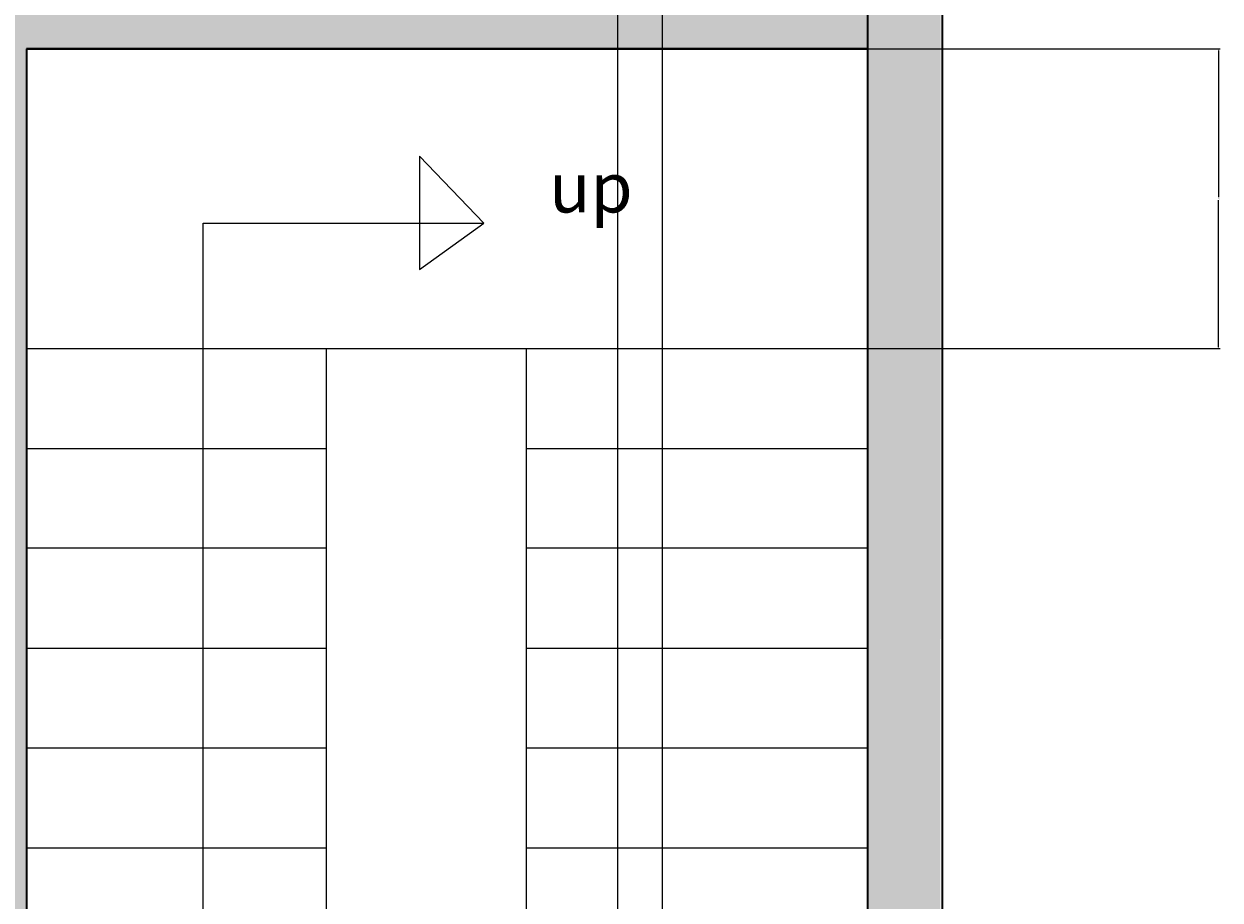
# Model space of a CAD drawing. Units: inches. Extents: x 2070 to 4408, y 1595 to 4269.
# Tile 8 of 20: x 2345 to 2489, y 1844 to 1949. Entities that reach past the tile are written whole.
import ezdxf

# ---------------------------------------------------------------- set-up
doc = ezdxf.new("R2010")
doc.units = ezdxf.units.IN
for name, color, linetype, lineweight in [('A-ANNO-DIMS', 2, 'Continuous', 18), ('A-ANNO-SYMB', 7, 'Continuous', 18), ('A-ANNO-TEXT', 7, 'Continuous', 18), ('A-FLOR-STRS', 7, 'Continuous', 18), ('A-WALL', 7, 'Continuous', 35)]:
    doc.layers.add(name, color=color, linetype=linetype, lineweight=lineweight)
doc.layers.add('A-WALL-PATT', color=18, linetype='Continuous', lineweight=13, true_color=0x000000)
doc.styles.get("Standard").update_dxf_attribs({"font": 'arial.ttf'})
doc.dimstyles.get("Standard").update_dxf_attribs({"dimtxt": 0.18, "dimasz": 0.18, "dimexe": 0.18, "dimexo": 0.0625, "dimgap": 0.09, "dimtad": 0, "dimtih": 1, "dimtoh": 1, "dimdec": 4, "dimzin": 0, "dimdsep": 46, "dimtxsty": 'Standard', "dimcen": 0.09, "dimadec": 0, "dimazin": 0, "dimtfac": 1, "dimtdec": 4, "dimtofl": 0, "dimtmove": 0, "dimatfit": 3, "dimfxl": 1, "dimtolj": 1, "dimtzin": 0, "dimarcsym": 0})

# ---------------------------------------------------------------- blocks, each defined once
blk = doc.blocks.new('*D30')
at = {"layer": 'A-ANNO-DIMS', "color": 0, "lineweight": -2, "transparency": 16777216}
for p, q in [((2416.2, 2080.34), (2416.2, 1595.04)), ((2446.2, 2080.34), (2446.2, 1595.04)), ((2416.38, 1595.22), (2430.98, 1595.22)), ((2446.02, 1595.22), (2431.41, 1595.22))]:
    blk.add_line(p, q, dxfattribs=at)
at = {"layer": 'A-ANNO-DIMS', "color": 0, "transparency": 16777216}
for points in [[(2416.38, 1595.25), (2416.38, 1595.19), (2416.2, 1595.22)], [(2446.02, 1595.25), (2446.02, 1595.19), (2446.2, 1595.22)]]:
    blk.add_solid(points, dxfattribs=at)
at = {"layer": 'Defpoints', "color": 0, "transparency": 16777216}
for p in [(2416.2, 2080.4), (2446.2, 2080.4), (2446.2, 1595.22)]:
    blk.add_point(p, dxfattribs=at)
at = {"layer": 'A-ANNO-DIMS', "color": 0, "transparency": 16777216, "insert": (2431.2, 1595.22), "char_height": 0.18, "attachment_point": 5}
blk.add_mtext('\\A1;30', dxfattribs=at)
blk = doc.blocks.new('*D34')
at = {"layer": 'A-ANNO-DIMS', "color": 0, "lineweight": -2, "transparency": 16777216}
for p, q in [((2421.53, 2212.34), (2421.53, 1595.04)), ((2446.2, 2212.34), (2446.2, 1595.04)), ((2421.71, 1595.22), (2433.4, 1595.22)), ((2446.02, 1595.22), (2434.33, 1595.22))]:
    blk.add_line(p, q, dxfattribs=at)
at = {"layer": 'A-ANNO-DIMS', "color": 0, "transparency": 16777216}
for points in [[(2421.71, 1595.25), (2421.71, 1595.19), (2421.53, 1595.22)], [(2446.02, 1595.25), (2446.02, 1595.19), (2446.2, 1595.22)]]:
    blk.add_solid(points, dxfattribs=at)
at = {"layer": 'Defpoints', "color": 0, "transparency": 16777216}
for p in [(2421.53, 2212.4), (2446.2, 2212.4), (2446.2, 1595.22)]:
    blk.add_point(p, dxfattribs=at)
at = {"layer": 'A-ANNO-DIMS', "color": 0, "transparency": 16777216, "insert": (2433.86, 1595.22), "char_height": 0.18, "attachment_point": 5}
blk.add_mtext('\\A1;24.663', dxfattribs=at)
blk = doc.blocks.new('*D41')
at = {"layer": 'A-ANNO-DIMS', "color": 0, "lineweight": -2, "transparency": 16777216}
for p, q in [((2446.26, 1946.4), (2488.56, 1946.4)), ((2488.38, 1946.22), (2488.38, 1928.58)), ((2488.38, 1910.58), (2488.38, 1928.22)), ((2446.26, 1910.4), (2488.56, 1910.4))]:
    blk.add_line(p, q, dxfattribs=at)
at = {"layer": 'A-ANNO-DIMS', "color": 0, "transparency": 16777216}
for points in [[(2488.35, 1946.22), (2488.41, 1946.22), (2488.38, 1946.4)], [(2488.35, 1910.58), (2488.41, 1910.58), (2488.38, 1910.4)]]:
    blk.add_solid(points, dxfattribs=at)
at = {"layer": 'Defpoints', "color": 0, "transparency": 16777216}
for p in [(2446.2, 1946.4), (2488.38, 1946.4), (2446.2, 1910.4)]:
    blk.add_point(p, dxfattribs=at)
at = {"layer": 'A-ANNO-DIMS', "color": 0, "transparency": 16777216, "insert": (2488.38, 1928.4), "char_height": 0.18, "attachment_point": 5}
blk.add_mtext('\\A1;36', dxfattribs=at)

msp = doc.modelspace()

# ---------------------------------------------------------------- hatches: boundary and pattern name
at = {"layer": 'A-WALL-PATT'}
h = msp.add_hatch(color=256, dxfattribs=at)
h.dxf.hatch_style = 1
h.paths.add_polyline_path([(2346.196, 2218.3995), (2346.196, 2282.3995), (2340.196, 2282.3995), (2340.196, 2212.3995), (2345.5866, 2212.3995), (2346.196, 2212.3995)], flags=0)
h.paths.add_polyline_path([(2245.196, 2282.3995), (2239.196, 2282.3995), (2239.196, 2186.3995), (2244.5866, 2186.3995), (2245.196, 2186.3995)], flags=0)
h.paths.add_polyline_path([(2340.196, 2230.6455), (2245.196, 2230.6455), (2245.196, 2224.6455), (2340.196, 2224.6455)], flags=0)
h.paths.add_polyline_path([(2245.196, 2150.3995), (2239.196, 2150.3995), (2164.4362, 2150.3995), (2164.4362, 2144.3995), (2239.196, 2144.3995), (2239.196, 2086.3995), (2239.196, 2067.2711), (2244.5866, 2067.2711), (2245.196, 2067.2711), (2245.196, 2144.3995)], flags=0)
h.paths.add_polyline_path([(2346.196, 2176.3995), (2340.196, 2176.3995), (2340.196, 2086.3995), (2346.196, 2086.3995), (2346.196, 2125.318)], flags=0)
h.paths.add_polyline_path([(2446.196, 2086.3995), (2346.196, 2086.3995), (2340.196, 2086.3995), (2340.196, 2080.3995), (2446.196, 2080.3995)], flags=0)
h.paths.add_polyline_path([(2455.196, 2291.3995), (2103.196, 2291.3995), (2103.196, 1699.3995), (2336.196, 1699.3995), (2336.196, 1628.3995), (2345.196, 1628.3995), (2446.196, 1628.3995), (2454.8846, 1628.3995), (2454.8846, 1699.3995)])
h.paths.add_polyline_path([(2446.196, 2282.3995), (2446.196, 2218.3995), (2446.196, 2212.3995), (2446.196, 2086.3995), (2446.196, 2080.3995), (2446.196, 1708.3995), (2446.196, 1637.3995), (2345.196, 1637.3995), (2345.196, 1699.3995), (2345.196, 1708.3995), (2336.196, 1708.3995), (2112.196, 1708.3995), (2112.196, 2282.3995), (2239.196, 2282.3995), (2245.196, 2282.3995), (2356.196, 2282.3995)], flags=16)
h.paths.add_polyline_path([(2245.196, 2150.3995), (2245.196, 2144.3995), (2245.196, 2067.2711), (2244.5866, 2067.2711), (2239.196, 2067.2711), (2239.196, 2065.6988), (2203.2929, 2065.6988, 0.40145271), (2239.196, 2031.3337), (2244.5866, 2031.3337), (2245.196, 2031.2711), (2245.196, 1924.1525), (2239.196, 1924.1525), (2239.196, 1922.5803), (2203.2929, 1922.5803, 0.40145271), (2239.196, 1888.2151), (2244.5866, 1888.2151), (2245.196, 1888.1525), (2245.196, 1748.3995), (2339.196, 1748.4621, -0.40145271), (2303.2929, 1782.8272), (2303.2585, 1782.8272), (2303.2585, 1784.3995), (2339.196, 1784.3995), (2339.196, 1877.2067), (2291.196, 1877.2067), (2291.196, 1883.2067), (2291.196, 1946.3995), (2291.196, 1952.3995), (2291.196, 2086.3995), (2297.196, 2086.3995), (2302.196, 2086.3995), (2302.196, 2081.0259), (2303.7633, 2081.0259), (2303.7633, 2080.3995), (2338.0148, 2080.3995, 0.00437129), (2338.0203, 2081.0259), (2338.0203, 2086.3995), (2340.196, 2086.3995), (2340.196, 2176.4621), (2345.5866, 2176.4621, 0.40145271), (2381.4896, 2210.8272), (2345.5866, 2210.8272), (2345.5866, 2212.3995), (2340.196, 2212.3995), (2340.196, 2224.6455), (2245.196, 2224.6455), (2245.196, 2186.3995), (2244.5866, 2186.3995), (2239.196, 2186.3995), (2239.196, 2184.8272), (2203.2929, 2184.8272, 0.40145271), (2239.196, 2150.4621), (2244.5866, 2150.4621)], flags=0)
h.paths.add_polyline_path([(2346.196, 2282.3995), (2346.196, 2218.3995), (2377.1813, 2218.3995), (2377.1813, 2212.3995), (2346.196, 2212.3995), (2345.5866, 2212.3995), (2340.196, 2212.3995), (2340.196, 2224.6455), (2245.196, 2224.6455), (2245.196, 2230.6455), (2245.196, 2282.3995), (2292.696, 2256.5225), (2340.196, 2282.3995)], flags=0)
h.paths.add_polyline_path([(2346.196, 2086.3995), (2340.196, 2086.3995), (2340.196, 2080.3995), (2446.196, 2080.3995), (2431.196, 2016.3995), (2446.196, 1952.3995), (2412.196, 1952.3995), (2412.196, 2080.3995), (2340.196, 2080.3995), (2340.196, 2086.3995), (2340.196, 2176.3995), (2346.196, 2176.3995), (2346.196, 2125.318)], flags=0)
h.paths.add_polyline_path([(2186.508, 2270.0471, -0.03755288), (2186.9712, 2269.8581), (2186.9164, 2270.112, -0.02759121)], flags=0)
h.paths.add_polyline_path([(2183.955, 2273.7766, 1), (2188.2945, 2273.7766, 1)], flags=0)
h.paths.add_polyline_path([(2142.5261, 2274.6158, -0.03707541), (2142.5672, 2275.1696), (2142.5672, 2276.826), (2119.8759, 2276.826), (2119.8759, 2263.0962), (2140.4332, 2263.0962), (2142.5672, 2263.0962), (2142.5672, 2274.0621, -0.03707541)], flags=0)
h.paths.add_polyline_path([(2209.8974, 2263.0962), (2209.8974, 2262.2079), (2190.8042, 2262.2079), (2190.8042, 2263.0962)], flags=0)
h.paths.add_polyline_path([(2210.6382, 2276.1833), (2210.6382, 2263.9844), (2190.2185, 2263.9844), (2190.2185, 2276.1833)], flags=0)
h.paths.add_polyline_path([(2188.4362, 2273.7766, -1), (2183.8133, 2273.7766, -1)], flags=0)
h.paths.add_polyline_path([(2245.196, 2150.3995), (2245.196, 2144.3995), (2245.196, 2067.2711), (2239.196, 2067.2711), (2239.196, 2080.3995), (2172.196, 2080.3995), (2172.196, 2000.3995), (2239.196, 2000.3995), (2239.196, 1940.3995), (2159.0187, 1940.3995), (2123.0187, 1940.3995), (2112.196, 1940.3995), (2112.196, 1946.3995), (2123.0187, 1946.3995), (2123.0187, 1982.2238), (2124.586, 1982.2238), (2124.586, 1982.1895, -0.40145271), (2158.8429, 1946.3995), (2159.0187, 1946.3995), (2239.196, 1946.3995), (2239.196, 1994.3995), (2112.196, 1994.3995), (2112.196, 2000.3995), (2139.196, 2040.3995), (2112.196, 2080.3995), (2112.196, 2086.3995), (2239.196, 2086.3995), (2239.196, 2144.3995), (2209.5809, 2144.3995), (2209.5809, 2136.3995), (2203.0809, 2136.3995), (2205.0809, 2130.3996, -0.70257121), (2199.081, 2116.3995, -0.70256205), (2193.0809, 2130.3994), (2195.0809, 2136.3995), (2192.0809, 2136.3995), (2192.0809, 2134.8995), (2189.0809, 2134.8995), (2189.0809, 2135.8995), (2191.0809, 2135.8995), (2191.0809, 2136.3995), (2188.5809, 2136.3995), (2188.5809, 2144.3995), (2164.2481, 2144.3995, -0.39385849), (2130.0035, 2109.5491), (2130.0035, 2109.5147), (2128.4362, 2109.5147), (2128.4362, 2144.3995), (2112.196, 2144.3995), (2112.196, 2150.3995), (2128.4362, 2150.3995), (2128.4362, 2150.7127), (2164.4362, 2150.7127), (2164.4362, 2150.3995), (2239.196, 2150.3995)], flags=0)
h.paths.add_polyline_path([(2188.2075, 2266.8735), (2188.2075, 2211.8632, -0.41421356), (2185.4833, 2209.1391), (2146.7995, 2209.1391, -0.41421356), (2144.0754, 2211.8632), (2144.0754, 2266.8735, -0.41421356), (2146.7995, 2269.5976), (2185.4833, 2269.5976, -0.41421356)], flags=0)
h.paths.add_polyline_path([(2185.0844, 2273.7766, -1), (2187.1651, 2273.7766, -1)], flags=0)
h.paths.add_polyline_path([(2182.0486, 2259.2932), (2168.0953, 2259.2932), (2168.0953, 2260.8424), (2163.7261, 2260.8424), (2163.7261, 2259.2932), (2149.7727, 2259.2932), (2149.7727, 2266.3352), (2163.7261, 2266.3352), (2163.7261, 2261.9839), (2168.0953, 2261.9839), (2168.0953, 2266.3352), (2182.0486, 2266.3352)], flags=0)
h.paths.add_polyline_path([(2148.2585, 2250.2051), (2153.0615, 2241.8861, 0.39807048)], flags=0)
h.paths.add_polyline_path([(2162.7572, 2247.2885), (2153.1461, 2241.7396), (2148.1083, 2250.4653), (2157.7194, 2256.0142)], flags=0)
h.paths.add_polyline_path([(2162.6726, 2247.4351, -0.39286196), (2157.8415, 2255.6313), (2157.6431, 2255.6313), (2157.8696, 2255.7541)], flags=0)
h.paths.add_polyline_path([(2164.2604, 2145.339), (2164.4362, 2144.3995), (2164.4362, 2150.3995), (2164.2604, 2150.7127)], flags=0)
h.paths.add_polyline_path([(2208.5809, 2142.6495), (2208.5809, 2138.3995, -0.41421356), (2207.8309, 2137.3995), (2190.5809, 2137.3995, -0.41421356), (2189.5809, 2138.1495), (2189.5809, 2142.3995, -0.41421356), (2190.3309, 2143.3995), (2207.5809, 2143.3995, -0.41421356)], flags=0)
h.paths.add_polyline_path([(2147.957, 2229.9119), (2154.7494, 2223.1195, 0.39807048)], flags=0)
h.paths.add_polyline_path([(2162.7165, 2230.8473), (2154.8691, 2222.9998), (2147.7446, 2230.1244), (2155.592, 2237.9718)], flags=0)
h.paths.add_polyline_path([(2162.5969, 2230.9669, -0.39807048), (2155.8044, 2237.7594)], flags=0)
h.paths.add_polyline_path([(2391.8776, 2049.9192), (2408.5766, 2049.9192), (2408.5766, 2033.2202), (2408.5766, 1983.123), (2408.5766, 1966.4239), (2391.8776, 1966.4239), (2391.8776, 1983.123), (2341.7804, 1983.123), (2341.7804, 2033.2202), (2391.8776, 2033.2202)], flags=0)
h.paths.add_polyline_path([(2144.1055, 2274.6158, 1), (2148.445, 2274.6158, 1)], flags=0)
h.paths.add_polyline_path([(2148.5867, 2274.6158, -1), (2143.9638, 2274.6158, -1)], flags=0)
h.paths.add_polyline_path([(2145.2349, 2274.6158, -1), (2147.3156, 2274.6158, -1)], flags=0)
edge = h.paths.add_edge_path(flags=0)
edge.add_ellipse((2400.5951, 2040.9436), major_axis=(-4.5109, 0), ratio=0.97544784, start_angle=180, end_angle=270, ccw=False)
edge.add_ellipse((2400.5951, 2040.9436), major_axis=(-4.5109, 0), ratio=0.97544784, start_angle=90, end_angle=180, ccw=False)
edge.add_ellipse((2400.5951, 2040.9436), major_axis=(-4.5109, 0), ratio=0.97544784, start_angle=0, end_angle=90, ccw=False)
edge.add_ellipse((2400.5951, 2040.9436), major_axis=(-4.5109, 0), ratio=0.97544784, start_angle=270, end_angle=360, ccw=False)
h.paths.add_polyline_path([(2199.0809, 2117.3995, -0.73452973), (2195.0809, 2130.3995), (2203.081, 2130.3995, -0.73453329)], flags=0)
h.paths.add_polyline_path([(2141.9147, 2276.0353), (2141.9147, 2263.9844), (2120.4685, 2263.9844), (2120.4685, 2276.0353)], flags=0)
h.paths.add_polyline_path([(2138.4481, 2273.4072), (2138.4481, 2266.7226), (2133.2801, 2266.7226), (2133.2801, 2273.4072)], flags=0)
h.paths.add_polyline_path([(2137.9691, 2272.9175), (2137.9691, 2272.204), (2135.4229, 2272.204), (2135.4229, 2271.6329), (2135.3221, 2270.1051), (2135.3221, 2269.0265), (2135.4229, 2268.6811), (2135.4229, 2267.2011), (2133.7212, 2267.2011), (2133.7212, 2268.6811), (2133.7983, 2269.9587), (2133.7983, 2271.2758), (2133.7212, 2271.6329), (2133.7212, 2273.0065), (2135.717, 2273.0065), (2135.717, 2272.9175)], flags=0)
h.paths.add_polyline_path([(2137.9215, 2271.8264), (2137.9215, 2271.3786), (2137.5182, 2271.3786), (2136.9355, 2271.3786), (2136.3529, 2271.3786), (2135.7703, 2271.3786), (2135.7703, 2271.8264), (2136.1736, 2271.8264), (2136.7562, 2271.8264), (2137.3389, 2271.8264)], flags=0)
h.paths.add_polyline_path([(2137.9215, 2271.692), (2137.5182, 2271.692), (2136.9355, 2271.513), (2137.3389, 2271.513)], flags=0)
h.paths.add_polyline_path([(2136.3529, 2271.692), (2135.7703, 2271.513), (2136.1736, 2271.513), (2136.7562, 2271.692)], flags=0)
h.paths.add_polyline_path([(2137.9215, 2271.513), (2137.5182, 2271.513), (2136.7562, 2271.747), (2136.7562, 2271.692), (2137.3389, 2271.692)], flags=0)
h.paths.add_polyline_path([(2137.8207, 2270.4664), (2137.8207, 2270.0971), (2137.8207, 2269.627), (2137.8207, 2269.1569), (2137.8207, 2268.6868), (2137.3837, 2268.6868), (2136.6442, 2268.6868), (2135.9271, 2268.6868), (2135.9271, 2269.0562), (2135.9271, 2269.5263), (2135.9271, 2269.9963), (2135.9271, 2270.4664), (2136.3641, 2270.4664), (2137.0812, 2270.4664)], flags=0)
h.paths.add_polyline_path([(2137.3837, 2269.627), (2137.8207, 2269.627), (2137.8207, 2269.5263), (2137.3837, 2269.5263), (2137.3837, 2269.1569), (2137.8207, 2269.1569), (2137.3837, 2269.0562), (2137.3837, 2268.6868), (2137.0812, 2268.6868), (2137.0812, 2269.0562), (2136.6442, 2269.0562), (2136.6442, 2268.6868), (2136.3641, 2268.6868), (2136.3641, 2269.0562), (2135.9271, 2269.0562), (2135.9271, 2269.1569), (2136.3641, 2269.1569), (2136.3641, 2269.5263), (2135.9271, 2269.5263), (2135.9271, 2269.627), (2136.3641, 2269.627), (2136.3641, 2269.9963), (2135.9271, 2269.9963), (2136.3641, 2270.0971), (2136.3641, 2270.4664), (2136.6442, 2270.4664), (2136.6442, 2270.0971), (2137.0812, 2270.0971), (2137.0812, 2270.4664), (2137.3837, 2270.4664), (2137.3837, 2270.0971), (2137.8207, 2270.0971), (2137.3837, 2269.9963)], flags=0)
h.paths.add_polyline_path([(2137.5182, 2271.8264), (2137.5182, 2271.692), (2137.3389, 2271.3786), (2137.3389, 2271.513)], flags=0)
h.paths.add_polyline_path([(2137.8179, 2267.8138), (2137.8179, 2267.6879), (2137.1876, 2267.6879), (2136.4733, 2267.6879), (2135.759, 2267.6879), (2135.759, 2267.8138), (2136.3893, 2267.8138), (2137.1036, 2267.8138)], flags=0)
h.paths.add_polyline_path([(2137.0812, 2269.9963), (2137.0812, 2269.627), (2137.0812, 2269.1569), (2136.6442, 2269.1569), (2136.6442, 2269.5263), (2136.6442, 2269.9963)], flags=0)
h.paths.add_polyline_path([(2136.3529, 2271.8264), (2136.3529, 2271.692), (2136.1736, 2271.3786), (2136.1736, 2271.513)], flags=0)
h.paths.add_polyline_path([(2136.4733, 2267.8138), (2136.4733, 2267.6879), (2136.3893, 2267.6879), (2136.3893, 2267.8138)], flags=0)
h.paths.add_polyline_path([(2407.9087, 2032.5522), (2407.9087, 1983.7909), (2359.81, 1983.7909, -0.00912788), (2359.0575, 1983.7909), (2342.4483, 1983.7909), (2342.4483, 2032.5522)], flags=0)
h.paths.add_polyline_path([(2389.1838, 2023.1358), (2353.7856, 2023.1358), (2353.7856, 1985.4867, -0.09210376), (2350.2788, 1988.655), (2350.2788, 2026.6426), (2389.1838, 2026.6426)], flags=0)
h.paths.add_polyline_path([(2352.6166, 2024.3048), (2351.4477, 2024.3048), (2351.4477, 2025.4737), (2352.6166, 2025.4737)], flags=0)
h.paths.add_polyline_path([(2399.6319, 2026.7589), (2404.3661, 2026.7589, -0.41421356), (2407.0379, 2024.087), (2407.0379, 2013.4908, -0.41421356), (2404.3661, 2010.819), (2399.6319, 2010.819, -0.41421356), (2396.96, 2013.4908), (2396.96, 2024.087, -0.41421356)], flags=0)
h.paths.add_polyline_path([(2399.6319, 2026.0909), (2404.3661, 2026.0909, -0.41421356), (2406.37, 2024.087), (2406.37, 2013.4908, -0.41421356), (2404.3661, 2011.487), (2399.6319, 2011.487, -0.41421356), (2397.628, 2013.4908), (2397.628, 2024.087, -0.41421356)], flags=0)
h.paths.add_polyline_path([(2399.6319, 2002.3217), (2404.3661, 2002.3217, -0.41421356), (2407.0379, 1999.6498), (2407.0379, 1989.0536, -0.41421356), (2404.3661, 1986.3818), (2399.6319, 1986.3818, -0.41421356), (2396.96, 1989.0536), (2396.96, 1999.6498, -0.41421356)], flags=0)
h.paths.add_polyline_path([(2399.6319, 2001.6537), (2404.3661, 2001.6537, -0.41421356), (2406.37, 1999.6498), (2406.37, 1989.0536, -0.41421356), (2404.3661, 1987.0497), (2399.6319, 1987.0497, -0.41421356), (2397.628, 1989.0536), (2397.628, 1999.6498, -0.41421356)], flags=0)
edge = h.paths.add_edge_path(flags=0)
edge.add_ellipse((2400.5951, 1975.3996), major_axis=(-4.5109, 0), ratio=0.97544784, start_angle=-180, end_angle=-90, ccw=False)
edge.add_ellipse((2400.5951, 1975.3996), major_axis=(-4.5109, 0), ratio=0.97544784, start_angle=90, end_angle=180, ccw=False)
edge.add_ellipse((2400.5951, 1975.3996), major_axis=(-4.5109, 0), ratio=0.97544784, start_angle=0, end_angle=90, ccw=False)
edge.add_ellipse((2400.5951, 1975.3996), major_axis=(-4.5109, 0), ratio=0.97544784, start_angle=-90, end_angle=0, ccw=False)
h.paths.add_polyline_path([(2345.196, 1910.3995), (2366.4386, 1910.3995), (2366.4386, 1925.4555), (2392.3856, 1925.4555), (2392.3856, 1933.5025), (2400.1399, 1925.4555), (2392.3856, 1919.8795), (2392.3856, 1925.4555), (2366.4386, 1925.4555), (2366.4386, 1910.3995), (2381.196, 1910.3995), (2405.196, 1910.3995), (2405.196, 1898.3995), (2446.196, 1898.3995), (2446.196, 1886.3995), (2405.196, 1886.3995), (2405.196, 1874.3995), (2446.196, 1874.3995), (2446.196, 1862.3995), (2405.196, 1862.3995), (2405.196, 1850.3995), (2446.196, 1850.3995), (2446.196, 1838.3995), (2405.196, 1838.3995), (2405.196, 1826.3995), (2446.196, 1826.3995), (2446.196, 1814.3995), (2405.196, 1814.3995), (2405.196, 1802.3995), (2446.196, 1802.3995), (2446.196, 1798.3995), (2446.196, 1792.3995), (2405.196, 1792.3995), (2405.196, 1910.3995), (2381.196, 1910.3995), (2381.196, 1792.3995), (2345.196, 1792.3995)], flags=0)
h.paths.add_polyline_path([(2333.0944, 1863.3993, -0.41421356), (2334.7225, 1861.7712), (2334.7225, 1859.329), (2335.2653, 1859.329, -0.41421356), (2337.4361, 1857.1582), (2337.4361, 1843.862, -0.41421356), (2335.2653, 1841.6911, -0.41421356), (2337.4361, 1839.5203), (2337.4361, 1827.5808, -0.41421356), (2335.2653, 1825.41, -0.41421356), (2337.4361, 1823.2392), (2337.4361, 1808.5862, -0.41421356), (2335.2653, 1806.4153), (2334.7225, 1806.4153), (2334.7225, 1803.9732, -0.41421356), (2333.0944, 1802.3451), (2317.356, 1802.3451), (2317.0846, 1802.3451, -0.41421356), (2315.7279, 1803.7018), (2315.7279, 1803.8646), (2313.8284, 1803.8646, -0.41421356), (2311.6576, 1806.0354), (2311.6576, 1823.2015, -0.39597602), (2313.6834, 1825.3765, -0.43384798), (2311.6576, 1827.2718), (2311.6576, 1839.761, -0.41421356), (2313.5571, 1841.6604), (2313.8284, 1841.6604), (2333.8159, 1841.6604, -0.04213623), (2334.1798, 1841.6911, -0.41421356), (2332.009, 1843.862), (2332.009, 1857.1582, -0.41421356), (2334.1798, 1859.329), (2317.356, 1859.329), (2317.0846, 1859.329, -0.41421356), (2315.7279, 1860.6858), (2315.7279, 1862.0426, -0.41421356), (2317.0846, 1863.3993), (2317.356, 1863.3993)], flags=0)
h.paths.add_polyline_path([(2208.8475, 1848.9818), (2208.8475, 1840.9741, -0.41421356), (2207.0458, 1839.1724), (2206.5453, 1839.1721), (2206.5453, 1838.7218, -0.40985861), (2204.7704, 1836.9203), (2183.7501, 1836.9203, -0.41858196), (2181.9216, 1838.7218), (2181.9216, 1839.1721), (2181.421, 1839.1724, -0.41421356), (2179.6193, 1840.9741), (2179.6193, 1848.6817, -0.44064415), (2185.1126, 1854.9874), (2203.3852, 1854.9874, -0.45707961)], flags=0)
h.paths.add_polyline_path([(2204.243, 1848.4815), (2204.243, 1848.4815, 0.41725335), (2202.2204, 1850.4833), (2186.2049, 1850.4833, 0.4111805), (2184.2237, 1848.4815), (2184.2237, 1848.4815, -0.4111807), (2186.2049, 1850.4833), (2202.2204, 1850.4833, -0.41725315)], flags=0)
h.paths.add_polyline_path([(2234.7177, 1830.228), (2234.7176, 1781.6047, -0.41421356), (2233.4381, 1780.3252), (2218.6064, 1780.3252, -0.41421356), (2217.8387, 1781.0929), (2217.8387, 1783.3961, -0.41421356), (2218.6064, 1784.1639), (2218.6065, 1796.9595, -0.41421356), (2219.886, 1798.239, -0.41421356), (2218.6065, 1799.5186), (2218.6065, 1812.3142, -0.41421356), (2219.8861, 1813.5938, -0.41421356), (2218.6065, 1814.8733), (2218.6065, 1827.6689, -0.41421356), (2217.8388, 1828.4367), (2217.8388, 1830.7399, -0.41421356), (2218.6065, 1831.5076), (2233.4382, 1831.5076, -0.41421356)], flags=0)
h.paths.add_polyline_path([(2230.6344, 1827.6689, -0.41421356), (2231.4021, 1826.9012), (2231.4021, 1784.9316, -0.41421356), (2230.6343, 1784.1639), (2221.1853, 1784.1639), (2221.1853, 1827.6689)], flags=0)
h.paths.add_polyline_path([(2222.7208, 1798.239), (2221.6971, 1798.239), (2221.6971, 1813.5938), (2222.7208, 1813.5938)], flags=0)
h.paths.add_polyline_path([(2206.5453, 1773.935), (2206.5453, 1773.4848), (2206.9457, 1773.4848), (2207.0458, 1773.4845, -0.41421356), (2208.8475, 1771.6827), (2208.8475, 1763.675, -0.44222432), (2203.6505, 1757.6695), (2185.3851, 1757.6695, -0.45508402), (2179.6193, 1763.9752), (2179.6193, 1771.6827, -0.41421356), (2181.421, 1773.4845), (2181.421, 1773.4848), (2181.9216, 1773.4848), (2181.9216, 1773.935, -0.40985861), (2183.6965, 1775.7366), (2204.7167, 1775.7366, -0.41858196)], flags=0)
h.paths.add_polyline_path([(2202.2619, 1762.1736), (2186.2464, 1762.1736, -0.41725315), (2184.2237, 1764.1754), (2184.2237, 1764.1754, 0.41725335), (2186.2464, 1762.1736), (2202.2619, 1762.1736, 0.4111805), (2204.243, 1764.1754), (2204.243, 1764.1754, -0.4111807)], flags=0)
h.paths.add_polyline_path([(2313.0034, 1713.1906), (2312.997, 1713.1697), (2313.0123, 1713.1612)], flags=0)
h.paths.add_polyline_path([(2305.7314, 1721.0488), (2305.6257, 1721.1994), (2305.4853, 1721.084)], flags=0)
h.paths.add_polyline_path([(2307.5562, 1726.1427), (2307.6186, 1726.1026), (2307.5737, 1726.0477), (2308.5692, 1720.6434), (2310.5345, 1721.2985), (2310.5721, 1721.411), (2310.6958, 1721.3523), (2313.8453, 1722.4021), (2314.9351, 1723.8033), (2314.9294, 1723.9165), (2315.0028, 1723.8903), (2313.874, 1722.4389), (2313.8697, 1722.4102), (2308.5692, 1720.6434), (2308.9864, 1720.122), (2309.0665, 1720.0971), (2309.053, 1720.0387), (2310.9235, 1717.7005), (2311.4182, 1717.6259), (2311.2918, 1717.2402), (2312.0655, 1716.2731), (2312.1081, 1716.2606), (2312.0969, 1716.2339), (2308.5692, 1720.6434), (2305.2249, 1717.745), (2305.232, 1717.704), (2305.1665, 1717.6944), (2308.5692, 1720.6434)], flags=0)
h.paths.add_polyline_path([(2288.2072, 1714.3431), (2288.2008, 1714.3222), (2288.216, 1714.3137)], flags=0)
h.paths.add_polyline_path([(2280.9352, 1722.2013), (2280.8295, 1722.3519), (2280.689, 1722.2365)], flags=0)
h.paths.add_polyline_path([(2282.76, 1727.2952), (2282.8224, 1727.2551), (2282.7775, 1727.2002), (2283.773, 1721.7959), (2285.7383, 1722.451), (2285.7759, 1722.5635), (2285.8995, 1722.5048), (2289.0491, 1723.5546), (2290.1389, 1724.9558), (2290.1332, 1725.069), (2290.2065, 1725.0428), (2289.0777, 1723.5915), (2289.0735, 1723.5628), (2283.773, 1721.7959), (2284.1901, 1721.2745), (2284.2703, 1721.2496), (2284.2567, 1721.1913), (2286.1273, 1718.8531), (2286.622, 1718.7785), (2286.4956, 1718.3927), (2287.2692, 1717.4256), (2287.3119, 1717.4131), (2287.3006, 1717.3864), (2283.773, 1721.7959), (2280.4286, 1718.8975), (2280.4357, 1718.8565), (2280.3703, 1718.8469), (2283.773, 1721.7959)], flags=0)
h.paths.add_polyline_path([(2302.0672, 1721.8694), (2301.8205, 1721.8572), (2301.7578, 1722.1787), (2299.415, 1724.5215), (2299.103, 1724.4694), (2299.0662, 1724.8703)], flags=0)
h.paths.add_polyline_path([(2264.5643, 1715.4956), (2264.5579, 1715.4747), (2264.5731, 1715.4662)], flags=0)
h.paths.add_polyline_path([(2257.2923, 1723.3538), (2257.1865, 1723.5044), (2257.0461, 1723.389)], flags=0)
h.paths.add_polyline_path([(2259.117, 1728.4477), (2259.1795, 1728.4077), (2259.1345, 1728.3527), (2260.13, 1722.9484), (2262.0954, 1723.6036), (2262.133, 1723.716), (2262.2566, 1723.6573), (2265.4061, 1724.7071), (2266.4959, 1726.1083), (2266.4902, 1726.2215), (2266.5636, 1726.1953), (2265.4348, 1724.744), (2265.4305, 1724.7153), (2260.13, 1722.9484), (2260.5472, 1722.427), (2260.6273, 1722.4022), (2260.6138, 1722.3438), (2262.4843, 1720.0056), (2262.979, 1719.931), (2262.8526, 1719.5452), (2263.6263, 1718.5781), (2263.6689, 1718.5656), (2263.6577, 1718.5389), (2260.13, 1722.9484), (2256.7857, 1720.05), (2256.7928, 1720.009), (2256.7273, 1719.9994), (2260.13, 1722.9484)], flags=0)
h.paths.add_polyline_path([(2277.2709, 1723.0219), (2277.0243, 1723.0097), (2276.9616, 1723.3312), (2274.6187, 1725.6741), (2274.3067, 1725.6219), (2274.27, 1726.0228)], flags=0)
h.paths.add_polyline_path([(2253.628, 1724.1744), (2253.3814, 1724.1622), (2253.3186, 1724.4838), (2250.9758, 1726.8266), (2250.6638, 1726.7744), (2250.627, 1727.1753)], flags=0)
h.paths.add_polyline_path([(2161.9194, 1715.4956), (2161.913, 1715.4747), (2161.9282, 1715.4662)], flags=0)
h.paths.add_polyline_path([(2154.6474, 1723.3538), (2154.5416, 1723.5044), (2154.4012, 1723.389)], flags=0)
h.paths.add_polyline_path([(2162.7899, 1724.744), (2162.7856, 1724.7153), (2157.4851, 1722.9484), (2157.9023, 1722.427), (2157.9824, 1722.4022), (2157.9689, 1722.3438), (2159.8394, 1720.0056), (2160.3341, 1719.931), (2160.2078, 1719.5452), (2160.9814, 1718.5781), (2161.024, 1718.5656), (2161.0128, 1718.5389), (2157.4851, 1722.9484), (2154.1408, 1720.05), (2154.1479, 1720.009), (2154.0824, 1719.9994), (2157.4851, 1722.9484), (2156.4721, 1728.4477), (2156.5346, 1728.4077), (2156.4896, 1728.3527), (2157.4851, 1722.9484), (2159.4505, 1723.6036), (2159.4881, 1723.716), (2159.6117, 1723.6573), (2162.7612, 1724.7071), (2163.851, 1726.1083), (2163.8453, 1726.2215), (2163.9187, 1726.1953)], flags=0)
h.paths.add_polyline_path([(2150.9831, 1724.1744), (2150.7365, 1724.1622), (2150.6738, 1724.4838), (2148.3309, 1726.8266), (2148.0189, 1726.7744), (2147.9822, 1727.1753)], flags=0)
h.paths.add_polyline_path([(2132.5099, 1716.6482), (2132.5035, 1716.6272), (2132.5187, 1716.6187)], flags=0)
h.paths.add_polyline_path([(2125.2379, 1724.5064), (2125.1322, 1724.6569), (2124.9917, 1724.5415)], flags=0)
h.paths.add_polyline_path([(2133.3804, 1725.8965), (2133.3762, 1725.8678), (2128.0757, 1724.101), (2128.4928, 1723.5795), (2128.5729, 1723.5547), (2128.5594, 1723.4963), (2130.43, 1721.1581), (2130.9246, 1721.0835), (2130.7983, 1720.6977), (2131.5719, 1719.7306), (2131.6146, 1719.7181), (2131.6033, 1719.6914), (2128.0757, 1724.101), (2124.7313, 1721.2025), (2124.7384, 1721.1615), (2124.6729, 1721.1519), (2128.0757, 1724.101), (2127.0626, 1729.6002), (2127.1251, 1729.5602), (2127.0801, 1729.5052), (2128.0757, 1724.101), (2130.041, 1724.7561), (2130.0786, 1724.8685), (2130.2022, 1724.8098), (2133.3517, 1725.8597), (2134.4415, 1727.2608), (2134.4358, 1727.3741), (2134.5092, 1727.3478)], flags=0)
h.paths.add_polyline_path([(2121.5736, 1725.3269), (2121.327, 1725.3148), (2121.2643, 1725.6363), (2118.9214, 1727.9791), (2118.6094, 1727.9269), (2118.5727, 1728.3279)], flags=0)
h.paths.add_polyline_path([(2433.3904, 1646.406), (2433.384, 1646.3851), (2433.3992, 1646.3766)], flags=0)
h.paths.add_polyline_path([(2426.1184, 1654.2642), (2426.0127, 1654.4148), (2425.8722, 1654.2994)], flags=0)
h.paths.add_polyline_path([(2427.9432, 1659.3581), (2428.0056, 1659.318), (2427.9606, 1659.2631), (2428.9562, 1653.8588), (2430.9215, 1654.514), (2430.9591, 1654.6264), (2431.0827, 1654.5677), (2434.2323, 1655.6175), (2435.322, 1657.0187), (2435.3163, 1657.1319), (2435.3897, 1657.1057), (2434.2609, 1655.6544), (2434.2567, 1655.6257), (2428.9562, 1653.8588), (2429.3733, 1653.3374), (2429.4534, 1653.3126), (2429.4399, 1653.2542), (2431.3105, 1650.916), (2431.8051, 1650.8414), (2431.6788, 1650.4556), (2432.4524, 1649.4885), (2432.4951, 1649.476), (2432.4838, 1649.4493), (2428.9562, 1653.8588), (2425.6118, 1650.9604), (2425.6189, 1650.9194), (2425.5535, 1650.9098), (2428.9562, 1653.8588)], flags=0)
h.paths.add_polyline_path([(2376.63, 1645.4912), (2376.6236, 1645.4703), (2376.6388, 1645.4617)], flags=0)
h.paths.add_polyline_path([(2369.358, 1653.3494), (2369.2523, 1653.5), (2369.1118, 1653.3845)], flags=0)
h.paths.add_polyline_path([(2371.1828, 1658.4432), (2371.2452, 1658.4032), (2371.2003, 1658.3482), (2372.1958, 1652.944), (2374.1611, 1653.5991), (2374.1987, 1653.7116), (2374.3224, 1653.6528), (2377.4719, 1654.7027), (2378.5617, 1656.1038), (2378.556, 1656.2171), (2378.6293, 1656.1908), (2377.5005, 1654.7395), (2377.4963, 1654.7108), (2372.1958, 1652.944), (2372.6129, 1652.4225), (2372.6931, 1652.3977), (2372.6795, 1652.3393), (2374.5501, 1650.0011), (2375.0448, 1649.9265), (2374.9184, 1649.5407), (2375.692, 1648.5737), (2375.7347, 1648.5611), (2375.7234, 1648.5344), (2372.1958, 1652.944), (2368.8514, 1650.0456), (2368.8586, 1650.0046), (2368.7931, 1649.995), (2372.1958, 1652.944)], flags=0)
h.paths.add_polyline_path([(2404.0947, 1645.0338), (2404.0883, 1645.0128), (2404.1035, 1645.0043)], flags=0)
h.paths.add_polyline_path([(2396.8227, 1652.892), (2396.717, 1653.0425), (2396.5765, 1652.9271)], flags=0)
h.paths.add_polyline_path([(2398.6475, 1657.9858), (2398.7099, 1657.9458), (2398.665, 1657.8908), (2399.6605, 1652.4866), (2401.6258, 1653.1417), (2401.6634, 1653.2541), (2401.7871, 1653.1954), (2404.9366, 1654.2453), (2406.0264, 1655.6464), (2406.0207, 1655.7596), (2406.094, 1655.7334), (2404.9652, 1654.2821), (2404.961, 1654.2534), (2399.6605, 1652.4866), (2400.0776, 1651.9651), (2400.1578, 1651.9403), (2400.1442, 1651.8819), (2402.0148, 1649.5437), (2402.5095, 1649.4691), (2402.3831, 1649.0833), (2403.1567, 1648.1162), (2403.1994, 1648.1037), (2403.1881, 1648.077), (2399.6605, 1652.4866), (2396.3162, 1649.5881), (2396.3233, 1649.5471), (2396.2578, 1649.5375), (2399.6605, 1652.4866)], flags=0)
h.paths.add_polyline_path([(2419.4532, 1658.0857), (2422.4541, 1655.0848), (2422.2075, 1655.0726), (2422.1448, 1655.3941), (2419.8019, 1657.737), (2419.4899, 1657.6848)], flags=0)
h.paths.add_polyline_path([(2390.1575, 1656.7135), (2393.1584, 1653.7125), (2392.9118, 1653.7004), (2392.8491, 1654.0219), (2390.5063, 1656.3647), (2390.1943, 1656.3125)], flags=0)
h.paths.add_polyline_path([(2362.6928, 1657.1709), (2365.6937, 1654.1699), (2365.4471, 1654.1578), (2365.3844, 1654.4793), (2363.0416, 1656.8221), (2362.7295, 1656.77)], flags=0)
h.paths.add_polyline_path([(2419.9523, 2037.8601), (2440.2872, 2037.8601), (2440.2872, 2047.1732), (2419.9523, 2047.1732)], flags=8)
h.paths.add_polyline_path([(2370.186, 1698.9005), (2413.6287, 1698.9005), (2413.6287, 1708.0908), (2370.186, 1708.0908)], flags=8)
h.paths.add_polyline_path([(2370.1656, 1708.5185), (2430.0857, 1708.5185), (2430.0857, 1717.8316), (2370.1656, 1717.8316)], flags=8)
h.paths.add_polyline_path([(2254.1469, 1788.1883), (2302.2471, 1788.1883), (2302.2471, 1797.3786), (2254.1469, 1797.3786)], flags=8)
h.paths.add_polyline_path([(2254.1264, 1797.8063), (2326.1448, 1797.8063), (2326.1448, 1807.1194), (2254.1264, 1807.1194)], flags=8)
h.paths.add_polyline_path([(2300.08, 1914.5069), (2338.861, 1914.5069), (2338.861, 1923.6972), (2300.08, 1923.6972)], flags=8)
h.paths.add_polyline_path([(2300.0595, 1924.1249), (2331.5882, 1924.1249), (2331.5882, 1933.438), (2300.0595, 1933.438)], flags=8)
h.paths.add_polyline_path([(2176.6905, 1716.4567), (2224.1441, 1716.4567), (2224.1441, 1725.647), (2176.6905, 1725.647)], flags=8)
h.paths.add_polyline_path([(2176.67, 1726.0747), (2245.9176, 1726.0747), (2245.9176, 1735.3878), (2176.67, 1735.3878)], flags=8)
h.paths.add_polyline_path([(2339.997, 2039.7696), (2388.1034, 2039.7696), (2388.1034, 2048.9661), (2339.997, 2048.9661)], flags=8)
h.paths.add_polyline_path([(2339.9776, 2049.3928), (2388.7204, 2049.3928), (2388.7204, 2058.7059), (2339.9776, 2058.7059)], flags=8)
h.paths.add_polyline_path([(2366.0063, 2161.3825), (2409.449, 2161.3825), (2409.449, 2170.5728), (2366.0063, 2170.5728)], flags=8)
h.paths.add_polyline_path([(2365.9868, 2171.0016), (2405.879, 2171.0016), (2405.879, 2180.3085), (2365.9868, 2180.3085)], flags=8)
h.paths.add_polyline_path([(2366.0102, 2247.0726), (2407.12, 2247.0726), (2407.12, 2256.263), (2366.0102, 2256.263)], flags=8)
h.paths.add_polyline_path([(2365.9897, 2256.6906), (2397.9686, 2256.6906), (2397.9686, 2266.0037), (2365.9897, 2266.0037)], flags=8)
h.paths.add_polyline_path([(2271.8465, 2102.7885), (2307.6541, 2102.7885), (2307.6541, 2111.9849), (2271.8465, 2111.9849)], flags=8)
h.paths.add_polyline_path([(2271.8281, 2112.4126), (2304.2673, 2112.4126), (2304.2673, 2121.7196), (2271.8281, 2121.7196)], flags=8)
h.paths.add_polyline_path([(2141.6408, 2187.5934), (2182.108, 2187.5934), (2182.108, 2196.7837), (2141.6408, 2196.7837)], flags=8)
h.paths.add_polyline_path([(2141.6203, 2197.2114), (2190.3631, 2197.2114), (2190.3631, 2206.5245), (2141.6203, 2206.5245)], flags=8)
h.paths.add_polyline_path([(2165.7271, 2103.039), (2211.5027, 2103.039), (2211.5027, 2112.2293), (2165.7271, 2112.2293)], flags=8)
h.paths.add_polyline_path([(2165.7077, 2112.658), (2185.1033, 2112.658), (2185.1033, 2121.965), (2165.7077, 2121.965)], flags=8)
h.paths.add_polyline_path([(2174.945, 2048.0789), (2211.3973, 2048.0789), (2211.3973, 2057.2693), (2174.945, 2057.2693)], flags=8)
h.paths.add_polyline_path([(2174.9256, 2057.698), (2194.3212, 2057.698), (2194.3212, 2067.0049), (2174.9256, 2067.0049)], flags=8)
h.paths.add_polyline_path([(2164.8305, 1965.8394), (2202.9649, 1965.8394), (2202.9649, 1975.0297), (2164.8305, 1975.0297)], flags=8)
h.paths.add_polyline_path([(2164.8111, 1975.4584), (2184.2067, 1975.4584), (2184.2067, 1984.7654), (2164.8111, 1984.7654)], flags=8)
h.paths.add_polyline_path([(2133.0392, 1862.086), (2173.5065, 1862.086), (2173.5065, 1871.2763), (2133.0392, 1871.2763)], flags=8)
h.paths.add_polyline_path([(2133.0709, 1871.8585), (2157.0382, 1871.8585), (2157.0382, 1880.8585), (2133.0709, 1880.8585)], flags=8)
h.paths.add_polyline_path([(2406.4423, 1923.5541), (2418.8209, 1923.5541), (2418.8209, 1932.7199), (2406.4423, 1932.7199)], flags=8)
h = msp.add_hatch(color=256, dxfattribs=at)
h.dxf.hatch_style = 1
h.paths.add_polyline_path([(2245.196, 2282.3995), (2239.196, 2282.3995), (2239.196, 2186.3995), (2244.5866, 2186.3995), (2245.196, 2186.3995)])
h.paths.add_polyline_path([(2340.196, 2230.6455), (2245.196, 2230.6455), (2245.196, 2224.6455), (2340.196, 2224.6455)])
h.paths.add_polyline_path([(2346.196, 2282.3995), (2340.196, 2282.3995), (2340.196, 2212.3995), (2345.5866, 2212.3995), (2346.196, 2212.3995), (2346.196, 2218.3995)])
h.paths.add_polyline_path([(2245.196, 2144.3995), (2245.196, 2150.3995), (2239.196, 2150.3995), (2164.4362, 2150.3995), (2164.4362, 2144.3995), (2239.196, 2144.3995), (2239.196, 2086.3995), (2239.196, 2067.2711), (2244.5866, 2067.2711), (2245.196, 2067.2711)])
h.paths.add_polyline_path([(2128.4362, 2150.3995), (2112.196, 2150.3995), (2112.196, 2144.3995), (2128.4362, 2144.3995), (2128.4362, 2145.339)])
h.paths.add_polyline_path([(2239.196, 2086.3995), (2112.196, 2086.3995), (2112.196, 2080.3995), (2239.196, 2080.3995)])
h.paths.add_polyline_path([(2172.196, 2080.3995), (2166.196, 2080.3995), (2166.196, 2000.3995), (2172.196, 2000.3995)])
h.paths.add_polyline_path([(2239.196, 2000.3995), (2112.196, 2000.3995), (2112.196, 1994.3995), (2239.196, 1994.3995)])
h.paths.add_polyline_path([(2245.196, 2031.2711), (2239.196, 2031.2711), (2239.196, 2000.3995), (2239.196, 1940.3995), (2245.196, 1940.3995)])
h.paths.add_polyline_path([(2239.196, 1946.3995), (2159.0187, 1946.3995), (2159.0187, 1940.3995), (2239.196, 1940.3995)])
h.paths.add_polyline_path([(2123.0187, 1946.3995), (2112.196, 1946.3995), (2112.196, 1940.3995), (2123.0187, 1940.3995)])
h.paths.add_polyline_path([(2377.1813, 2218.3995), (2346.196, 2218.3995), (2346.196, 2212.3995), (2377.1813, 2212.3995)])
h.paths.add_polyline_path([(2446.196, 2218.3995), (2413.1813, 2218.3995), (2413.1813, 2212.3995), (2446.196, 2212.3995)])
h.paths.add_polyline_path([(2446.196, 2086.3995), (2346.196, 2086.3995), (2340.196, 2086.3995), (2340.196, 2080.3995), (2446.196, 2080.3995)], flags=17)
h.paths.add_polyline_path([(2346.196, 2125.318), (2346.196, 2176.3995), (2340.196, 2176.3995), (2340.196, 2086.3995), (2346.196, 2086.3995)])
h.paths.add_polyline_path([(2245.196, 1888.1525), (2239.196, 1888.1525), (2239.196, 1748.3995), (2245.196, 1748.3995)])
h.paths.add_polyline_path([(2345.196, 1748.3995), (2239.196, 1748.3995), (2112.196, 1748.3995), (2112.196, 1742.3995), (2239.196, 1742.3995), (2345.196, 1742.3995)])
h.paths.add_polyline_path([(2297.196, 2080.3995), (2297.196, 2086.3995), (2291.196, 2086.3995), (2291.196, 1952.3995), (2291.196, 1946.3995), (2339.196, 1946.3995), (2339.196, 1883.2067), (2291.196, 1883.2067), (2291.196, 1877.2067), (2339.196, 1877.2067), (2339.196, 1784.3995), (2345.196, 1784.3995), (2345.196, 1792.3995), (2345.196, 1946.3995), (2446.196, 1946.3995), (2446.196, 1952.3995), (2297.196, 1952.3995)])

# ---------------------------------------------------------------- linework, layer by layer
at = {"layer": 'A-ANNO-SYMB'}
for p, q in [((2400.1399, 1925.4555), (2392.3856, 1933.5025)), ((2392.3856, 1933.5025), (2392.3856, 1925.4555)), ((2366.4386, 1778.524), (2366.4386, 1925.4555)), ((2366.4386, 1925.4555), (2400.1399, 1925.4555)), ((2392.3856, 1925.4555), (2392.3856, 1919.8795)), ((2392.3856, 1919.8795), (2400.1399, 1925.4555))]:
    msp.add_line(p, q, dxfattribs=at)
at = {"layer": 'A-FLOR-STRS'}
for p, q in [((2345.196, 1946.3995), (2345.196, 1910.3995)), ((2345.196, 1910.3995), (2446.196, 1910.3995)), ((2345.196, 1910.3995), (2381.196, 1910.3995)), ((2345.196, 1910.3995), (2345.196, 1898.3995)), ((2381.196, 1910.3995), (2381.196, 1792.3995)), ((2381.196, 1910.3995), (2405.196, 1910.3995)), ((2405.196, 1910.3995), (2405.196, 1792.3995)), ((2345.196, 1898.3995), (2381.196, 1898.3995)), ((2405.196, 1898.3995), (2446.196, 1898.3995)), ((2446.196, 1898.3995), (2446.196, 1886.3995)), ((2345.196, 1886.3995), (2345.196, 1874.3995)), ((2381.196, 1886.3995), (2345.196, 1886.3995)), ((2446.196, 1886.3995), (2405.196, 1886.3995)), ((2345.196, 1874.3995), (2381.196, 1874.3995)), ((2405.196, 1874.3995), (2446.196, 1874.3995)), ((2446.196, 1874.3995), (2446.196, 1862.3995)), ((2345.196, 1862.3995), (2345.196, 1862.3995)), ((2345.196, 1862.3995), (2345.196, 1850.3995)), ((2381.196, 1862.3995), (2345.196, 1862.3995)), ((2446.196, 1862.3995), (2405.196, 1862.3995)), ((2345.196, 1850.3995), (2381.196, 1850.3995)), ((2405.196, 1850.3995), (2446.196, 1850.3995)), ((2446.196, 1850.3995), (2446.196, 1850.3995)), ((2446.196, 1850.3995), (2446.196, 1838.3995))]:
    msp.add_line(p, q, dxfattribs=at)
at = {"layer": 'A-WALL'}
for p, q in [((2446.196, 1946.3995), (2345.196, 1946.3995)), ((2345.196, 1946.3995), (2345.196, 1784.3995)), ((2345.196, 1946.3995), (2446.196, 1946.3995))]:
    msp.add_line(p, q, dxfattribs=at)
for points in [[(2336.196, 1699.3995), (2103.196, 1699.3995), (2103.196, 2291.3995), (2455.196, 2291.3995), (2455.196, 1699.3995), (2454.8846, 1699.3995)], [(2446.196, 2212.3995), (2446.196, 1708.3995)]]:
    msp.add_lwpolyline(points, dxfattribs=at)

# ---------------------------------------------------------------- texts
at = {"layer": 'A-ANNO-TEXT'}
msp.add_text('up', height=6, dxfattribs=at).set_placement((2407.9699, 1926.7475))

# ---------------------------------------------------------------- dimensions: what is measured, and where the dimension line sits
at = {"layer": 'A-ANNO-DIMS'}
for p1, p2, override, picture, middle in [((2421.5333, 2212.3995), (2446.196, 2212.3995), {"dimdec": 3, "dimlfac": 1, "dimrnd": 0, "dimzin": 0, "dimdsep": 46, "dimlunit": 2}, '*D34', (2433.8646, 1595.2195)), ((2416.196, 2080.3995), (2446.196, 2080.3995), {"dimdec": 0, "dimlfac": 1, "dimrnd": 0, "dimzin": 0, "dimdsep": 46, "dimlunit": 2}, '*D30', (2431.196, 1595.2195))]:
    dim = msp.add_linear_dim(base=(2446.196, 1595.2195), p1=p1, p2=p2, dimstyle='Standard', override=override, dxfattribs=at)
    dim.commit()
    dim.dimension.update_dxf_attribs({"geometry": picture, "text_midpoint": middle})
dim = msp.add_linear_dim(base=(2488.376, 1946.3995), p1=(2446.196, 1910.3995), p2=(2446.196, 1946.3995), angle=90, dimstyle='Standard', override={"dimdec": 0, "dimlfac": 1, "dimrnd": 0, "dimzin": 0, "dimdsep": 46, "dimlunit": 2}, dxfattribs=at)
dim.commit()
dim.dimension.update_dxf_attribs({"geometry": '*D41', "text_midpoint": (2488.376, 1928.3995)})

doc.saveas('drawing.dxf')
